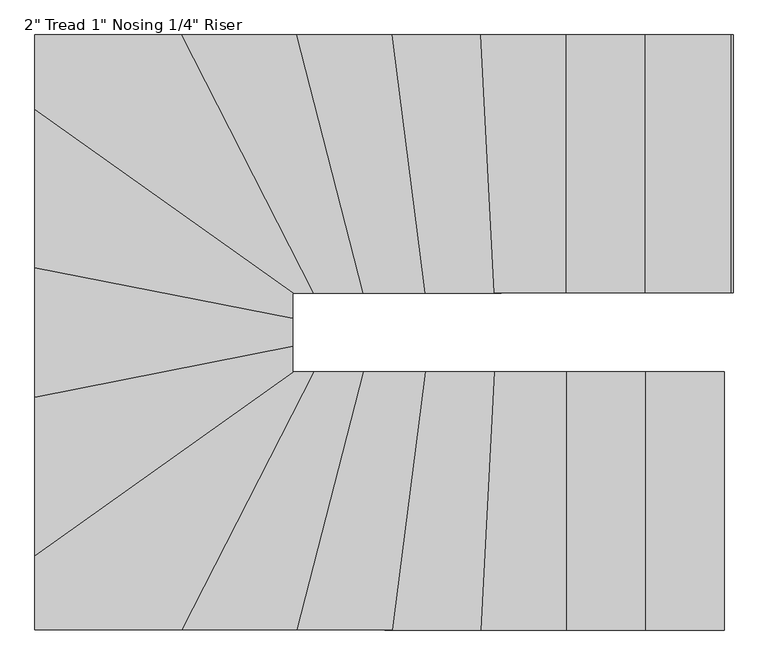
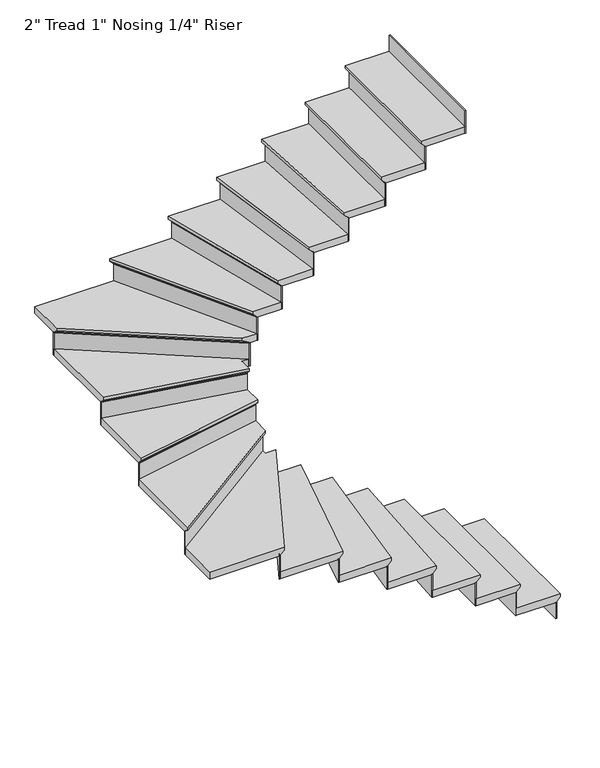
"""IFC4 building model written with IfcOpenShell, lengths in millimetres: stair flight geometry."""

from ifc_helpers import new_model, si_unit, origin, place, context, project, spatial, faceted_brep, source, transform, mapped, element, save


def stair_flight_e257120f(model_context):
    return source(origin(), model_context, "Body", "Brep", [
        faceted_brep([(-1783.4132248, -345.7070853, 3350.6833333), (-1783.4132248, -345.7070853, 3369.7333333), (-1783.4132248, -1260.1070853, 3369.7333333), (-1783.4132248, -1260.1070853, 3350.6833333), (-1808.8132248, -345.7070853, 3325.2833333), (-1808.8132248, -1260.1070853, 3325.2833333), (-2088.2132248, -345.7070853, 3369.7333333), (-2088.2132248, -1260.1070853, 3369.7333333), (-1808.8132248, -1260.1070853, 3318.9333333), (-2088.2132248, -1260.1070853, 3318.9333333), (-2088.2132248, -345.7070853, 3318.9333333), (-1808.8132248, -345.7070853, 3318.9333333)], [[[0, 1, 2, 3]], [[4, 0, 3, 5]], [[2, 1, 6, 7]], [[8, 9, 10, 11]], [[2, 7, 9, 8, 5, 3]], [[8, 11, 4, 5]], [[6, 1, 0, 4, 11, 10]], [[7, 6, 10, 9]]]),
        faceted_brep([(-1808.8132248, -345.7070853, 3318.9333333), (-1808.8132248, -345.7070853, 3200.4), (-1815.1632248, -345.7070853, 3200.4), (-1815.1632248, -345.7070853, 3318.9333333), (-1808.8132248, -1260.1070853, 3318.9333333), (-1815.1632248, -1260.1070853, 3318.9333333), (-1815.1632248, -1260.1070853, 3200.4), (-1808.8132248, -1260.1070853, 3200.4)], [[[0, 1, 2, 3]], [[4, 5, 6, 7]], [[1, 0, 4, 7]], [[2, 1, 7, 6]], [[3, 2, 6, 5]], [[0, 3, 5, 4]]]),
        faceted_brep([(-2088.2132248, -345.7070853, 3488.2666667), (-2088.2132248, -345.7070853, 3318.9333333), (-2094.5632248, -345.7070853, 3318.9333333), (-2094.5632248, -345.7070853, 3488.2666667), (-2088.2132248, -1260.1070853, 3488.2666667), (-2094.5632248, -1260.1070853, 3488.2666667), (-2094.5632248, -1260.1070853, 3318.9333333), (-2088.2132248, -1260.1070853, 3318.9333333)], [[[0, 1, 2, 3]], [[4, 5, 6, 7]], [[1, 0, 4, 7]], [[2, 1, 7, 6]], [[3, 2, 6, 5]], [[0, 3, 5, 4]]]),
        faceted_brep([(-2062.8132248, -1260.1070853, 3539.0666667), (-2062.8132248, -345.7070853, 3539.0666667), (-2367.6132248, -345.7070853, 3539.0666667), (-2367.6132248, -1260.1070853, 3539.0666667), (-2088.2132248, -1260.1070853, 3488.2666667), (-2367.6132248, -1260.1070853, 3488.2666667), (-2367.6132248, -345.7070853, 3488.2666667), (-2088.2132248, -345.7070853, 3488.2666667), (-2088.2132248, -1260.1070853, 3494.6166667), (-2062.8132248, -1260.1070853, 3520.0166667), (-2088.2132248, -345.7070853, 3494.6166667), (-2062.8132248, -345.7070853, 3520.0166667)], [[[0, 1, 2, 3]], [[4, 5, 6, 7]], [[0, 3, 5, 4, 8, 9]], [[4, 7, 10, 8]], [[2, 1, 11, 10, 7, 6]], [[3, 2, 6, 5]], [[11, 1, 0, 9]], [[10, 11, 9, 8]]]),
        faceted_brep([(-2367.6132248, -345.7070853, 3657.6), (-2367.6132248, -345.7070853, 3488.2666667), (-2373.9632248, -345.7070853, 3488.2666667), (-2373.9632248, -345.7070853, 3657.6), (-2367.6132248, -1260.1070853, 3657.6), (-2373.9632248, -1260.1070853, 3657.6), (-2373.9632248, -1260.1070853, 3488.2666667), (-2367.6132248, -1260.1070853, 3488.2666667)], [[[0, 1, 2, 3]], [[4, 5, 6, 7]], [[1, 0, 4, 7]], [[2, 1, 7, 6]], [[3, 2, 6, 5]], [[0, 3, 5, 4]]]),
        faceted_brep([(-2342.2132248, -1260.1070853, 3708.4), (-2342.2132248, -345.7070853, 3708.4), (-2623.2803863, -345.7070853, 3708.4), (-2670.8146567, -1260.1070853, 3708.4), (-2367.6132248, -1260.1070853, 3657.6), (-2670.8146567, -1260.1070853, 3657.6), (-2623.2803863, -345.7070853, 3657.6), (-2367.6132248, -345.7070853, 3657.6), (-2367.6132248, -1260.1070853, 3663.95), (-2342.2132248, -1260.1070853, 3689.35), (-2367.6132248, -345.7070853, 3663.95), (-2342.2132248, -345.7070853, 3689.35)], [[[0, 1, 2, 3]], [[4, 5, 6, 7]], [[0, 3, 5, 4, 8, 9]], [[4, 7, 10, 8]], [[2, 1, 11, 10, 7, 6]], [[3, 2, 6, 5]], [[11, 1, 0, 9]], [[10, 11, 9, 8]]]),
        faceted_brep([(-2623.2803863, -345.7070853, 3826.9333333), (-2623.2803863, -345.7070853, 3657.6), (-2629.6389604, -345.7070853, 3657.6), (-2629.6389604, -345.7070853, 3826.9333333), (-2670.8146567, -1260.1070853, 3826.9333333), (-2677.1732308, -1260.1070853, 3826.9333333), (-2677.1732308, -1260.1070853, 3657.6), (-2670.8146567, -1260.1070853, 3657.6)], [[[0, 1, 2, 3]], [[4, 5, 6, 7]], [[1, 0, 4, 7]], [[2, 1, 7, 6]], [[3, 2, 6, 5]], [[0, 3, 5, 4]]]),
        faceted_brep([(-2645.38036, -1260.1070853, 3877.7333333), (-2597.8460896, -345.7070853, 3877.7333333), (-2867.4470861, -345.7070853, 3877.7333333), (-2985.8031378, -1260.1070853, 3877.7333333), (-2670.8146567, -1260.1070853, 3826.9333333), (-2985.8031378, -1260.1070853, 3826.9333333), (-2867.4470861, -345.7070853, 3826.9333333), (-2623.2803863, -345.7070853, 3826.9333333), (-2670.8146567, -1260.1070853, 3833.2833333), (-2645.38036, -1260.1070853, 3858.6833333), (-2623.2803863, -345.7070853, 3833.2833333), (-2597.8460896, -345.7070853, 3858.6833333)], [[[0, 1, 2, 3]], [[4, 5, 6, 7]], [[0, 3, 5, 4, 8, 9]], [[4, 7, 10, 8]], [[2, 1, 11, 10, 7, 6]], [[3, 2, 6, 5]], [[11, 1, 0, 9]], [[10, 11, 9, 8]]]),
        faceted_brep([(-2867.4470861, -345.7070853, 3996.2666667), (-2867.4470861, -345.7070853, 3826.9333333), (-2873.8500579, -345.7070853, 3826.9333333), (-2873.8500579, -345.7070853, 3996.2666667), (-2985.8031378, -1260.1070853, 3996.2666667), (-2992.2061095, -1260.1070853, 3996.2666667), (-2992.2061095, -1260.1070853, 3826.9333333), (-2985.8031378, -1260.1070853, 3826.9333333)], [[[0, 1, 2, 3]], [[4, 5, 6, 7]], [[1, 0, 4, 7]], [[2, 1, 7, 6]], [[3, 2, 6, 5]], [[0, 3, 5, 4]]]),
        faceted_brep([(-2960.1912506, -1260.1070853, 4047.0666667), (-2841.835199, -345.7070853, 4047.0666667), (-3089.0743086, -345.7070853, 4047.0666667), (-3324.204756, -1260.1070853, 4047.0666667), (-2985.8031378, -1260.1070853, 3996.2666667), (-3324.204756, -1260.1070853, 3996.2666667), (-3089.0743086, -345.7070853, 3996.2666667), (-2867.4470861, -345.7070853, 3996.2666667), (-2985.8031378, -1260.1070853, 4002.6166667), (-2960.1912506, -1260.1070853, 4028.0166667), (-2867.4470861, -345.7070853, 4002.6166667), (-2841.835199, -345.7070853, 4028.0166667)], [[[0, 1, 2, 3]], [[4, 5, 6, 7]], [[0, 3, 5, 4, 8, 9]], [[4, 7, 10, 8]], [[2, 1, 11, 10, 7, 6]], [[3, 2, 6, 5]], [[11, 1, 0, 9]], [[10, 11, 9, 8]]]),
        faceted_brep([(-3089.0743086, -345.7070853, 4165.6), (-3089.0743086, -345.7070853, 3996.2666667), (-3095.6308854, -345.7070853, 3996.2666667), (-3095.6308854, -345.7070853, 4165.6), (-3324.204756, -1260.1070853, 4165.6), (-3330.7613329, -1260.1070853, 4165.6), (-3330.7613329, -1260.1070853, 3996.2666667), (-3324.204756, -1260.1070853, 3996.2666667)], [[[0, 1, 2, 3]], [[4, 5, 6, 7]], [[1, 0, 4, 7]], [[2, 1, 7, 6]], [[3, 2, 6, 5]], [[0, 3, 5, 4]]]),
        faceted_brep([(-3297.9784485, -1260.1070853, 4216.4), (-3062.8480011, -345.7070853, 4216.4), (-3265.4209447, -345.7070853, 4216.4), (-3734.245566, -1260.1070853, 4216.4), (-3324.204756, -1260.1070853, 4165.6), (-3734.245566, -1260.1070853, 4165.6), (-3265.4209447, -345.7070853, 4165.6), (-3089.0743086, -345.7070853, 4165.6), (-3324.204756, -1260.1070853, 4171.95), (-3297.9784485, -1260.1070853, 4197.35), (-3089.0743086, -345.7070853, 4171.95), (-3062.8480011, -345.7070853, 4197.35)], [[[0, 1, 2, 3]], [[4, 5, 6, 7]], [[0, 3, 5, 4, 8, 9]], [[4, 7, 10, 8]], [[2, 1, 11, 10, 7, 6]], [[3, 2, 6, 5]], [[11, 1, 0, 9]], [[10, 11, 9, 8]]]),
        faceted_brep([(-3265.4209447, -345.7070853, 4334.9333333), (-3265.4209447, -345.7070853, 4165.6), (-3272.5569278, -345.7070853, 4165.6), (-3272.5569278, -345.7070853, 4334.9333333), (-3734.245566, -1260.1070853, 4334.9333333), (-3741.3815491, -1260.1070853, 4334.9333333), (-3741.3815491, -1260.1070853, 4165.6), (-3734.245566, -1260.1070853, 4165.6)], [[[0, 1, 2, 3]], [[4, 5, 6, 7]], [[1, 0, 4, 7]], [[2, 1, 7, 6]], [[3, 2, 6, 5]], [[0, 3, 5, 4]]]),
        faceted_brep([(-4225.5449167, -966.4259516, 4385.7333333), (-4225.5449167, -1260.1070853, 4385.7333333), (-3705.7016335, -1260.1070853, 4385.7333333), (-3236.8770121, -345.7070853, 4385.7333333), (-3311.1449167, -345.7070853, 4385.7333333), (-3311.1449167, -316.1520025, 4385.7333333), (-4225.5449167, -1260.1070853, 4334.9333333), (-4225.5449167, -966.4259516, 4334.9333333), (-3311.1449167, -316.1520025, 4334.9333333), (-3311.1449167, -345.7070853, 4334.9333333), (-3265.4209447, -345.7070853, 4334.9333333), (-3734.245566, -1260.1070853, 4334.9333333), (-3734.245566, -1260.1070853, 4341.2833333), (-3705.7016335, -1260.1070853, 4366.6833333), (-3265.4209447, -345.7070853, 4341.2833333), (-3236.8770121, -345.7070853, 4366.6833333)], [[[0, 1, 2, 3, 4, 5]], [[6, 7, 8, 9, 10, 11]], [[1, 0, 7, 6]], [[2, 1, 6, 11, 12, 13]], [[11, 10, 14, 12]], [[4, 3, 15, 14, 10, 9]], [[5, 4, 9, 8]], [[0, 5, 8, 7]], [[15, 3, 2, 13]], [[14, 15, 13, 12]]]),
        faceted_brep([(-3311.1449167, -316.1520025, 4504.2666667), (-3311.1449167, -316.1520025, 4334.9333333), (-3311.1449167, -308.3600277, 4334.9333333), (-3311.1449167, -308.3600277, 4504.2666667), (-4225.5449167, -966.4259516, 4504.2666667), (-4225.5449167, -958.6339768, 4504.2666667), (-4225.5449167, -958.6339768, 4334.9333333), (-4225.5449167, -966.4259516, 4334.9333333)], [[[0, 1, 2, 3]], [[4, 5, 6, 7]], [[1, 0, 4, 7]], [[2, 1, 7, 6]], [[3, 2, 6, 5]], [[0, 3, 5, 4]]]),
        faceted_brep([(-4225.5449167, -997.5938508, 4555.0666667), (-3311.1449167, -347.3199017, 4555.0666667), (-3311.1449167, -229.6979154, 4555.0666667), (-4225.5449167, -409.9387717, 4555.0666667), (-4225.5449167, -966.4259516, 4504.2666667), (-4225.5449167, -409.9387717, 4504.2666667), (-3311.1449167, -229.6979154, 4504.2666667), (-3311.1449167, -316.1520025, 4504.2666667), (-4225.5449167, -966.4259516, 4510.6166667), (-4225.5449167, -997.5938508, 4536.0166667), (-3311.1449167, -316.1520025, 4510.6166667), (-3311.1449167, -347.3199017, 4536.0166667)], [[[0, 1, 2, 3]], [[4, 5, 6, 7]], [[0, 3, 5, 4, 8, 9]], [[4, 7, 10, 8]], [[2, 1, 11, 10, 7, 6]], [[3, 2, 6, 5]], [[11, 1, 0, 9]], [[10, 11, 9, 8]]]),
        faceted_brep([(-3311.1449167, -229.6979154, 4673.6), (-3311.1449167, -229.6979154, 4504.2666667), (-3311.1449167, -223.22573, 4504.2666667), (-3311.1449167, -223.22573, 4673.6), (-4225.5449167, -409.9387717, 4673.6), (-4225.5449167, -403.4665863, 4673.6), (-4225.5449167, -403.4665863, 4504.2666667), (-4225.5449167, -409.9387717, 4504.2666667)], [[[0, 1, 2, 3]], [[4, 5, 6, 7]], [[1, 0, 4, 7]], [[2, 1, 7, 6]], [[3, 2, 6, 5]], [[0, 3, 5, 4]]]),
        faceted_brep([(-4225.5449167, -435.8275135, 4724.4), (-3311.1449167, -255.5866572, 4724.4), (-3311.1449167, -130.5387717, 4724.4), (-4225.5449167, 49.7020846, 4724.4), (-4225.5449167, -409.9387717, 4673.6), (-4225.5449167, 49.7020846, 4673.6), (-3311.1449167, -130.5387717, 4673.6), (-3311.1449167, -229.6979154, 4673.6), (-4225.5449167, -409.9387717, 4679.95), (-4225.5449167, -435.8275135, 4705.35), (-3311.1449167, -229.6979154, 4679.95), (-3311.1449167, -255.5866572, 4705.35)], [[[0, 1, 2, 3]], [[4, 5, 6, 7]], [[0, 3, 5, 4, 8, 9]], [[4, 7, 10, 8]], [[2, 1, 11, 10, 7, 6]], [[3, 2, 6, 5]], [[11, 1, 0, 9]], [[10, 11, 9, 8]]]),
        faceted_brep([(-3311.1449167, -130.5387717, 4842.9333333), (-3311.1449167, -130.5387717, 4673.6), (-3311.1449167, -124.0665863, 4673.6), (-3311.1449167, -124.0665863, 4842.9333333), (-4225.5449167, 49.7020846, 4842.9333333), (-4225.5449167, 56.17427, 4842.9333333), (-4225.5449167, 56.17427, 4673.6), (-4225.5449167, 49.7020846, 4673.6)], [[[0, 1, 2, 3]], [[4, 5, 6, 7]], [[1, 0, 4, 7]], [[2, 1, 7, 6]], [[3, 2, 6, 5]], [[0, 3, 5, 4]]]),
        faceted_brep([(-4225.5449167, 23.8133428, 4893.7333333), (-3311.1449167, -156.4275135, 4893.7333333), (-3311.1449167, -66.3070853, 4893.7333333), (-3265.0494422, -66.3070853, 4893.7333333), (-4225.5449167, 616.7475793, 4893.7333333), (-4225.5449167, 49.7020846, 4842.9333333), (-4225.5449167, 616.7475793, 4842.9333333), (-3265.0494422, -66.3070853, 4842.9333333), (-3311.1449167, -66.3070853, 4842.9333333), (-3311.1449167, -130.5387717, 4842.9333333), (-4225.5449167, 49.7020846, 4849.2833333), (-4225.5449167, 23.8133428, 4874.6833333), (-3311.1449167, -130.5387717, 4849.2833333), (-3311.1449167, -156.4275135, 4874.6833333)], [[[0, 1, 2, 3, 4]], [[5, 6, 7, 8, 9]], [[0, 4, 6, 5, 10, 11]], [[5, 9, 12, 10]], [[2, 1, 13, 12, 9, 8]], [[3, 2, 8, 7]], [[4, 3, 7, 6]], [[13, 1, 0, 11]], [[12, 13, 11, 10]]]),
        faceted_brep([(-3265.0494422, -66.3070853, 5012.2666667), (-3265.0494422, -66.3070853, 4842.9333333), (-3254.0925497, -66.3070853, 4842.9333333), (-3254.0925497, -66.3070853, 5012.2666667), (-4225.5449167, 616.7475793, 5012.2666667), (-4225.5449167, 624.5395541, 5012.2666667), (-4225.5449167, 624.5395541, 4842.9333333), (-4225.5449167, 616.7475793, 4842.9333333)], [[[0, 1, 2, 3]], [[4, 5, 6, 7]], [[1, 0, 4, 7]], [[2, 1, 7, 6]], [[3, 2, 6, 5]], [[0, 3, 5, 4]]]),
        faceted_brep([(-3677.1577009, 848.0929147, 5063.0666667), (-4225.5449167, 848.0929147, 5063.0666667), (-4225.5449167, 585.5796802, 5063.0666667), (-3308.8770121, -66.3070853, 5063.0666667), (-3208.3330796, -66.3070853, 5063.0666667), (-4225.5449167, 848.0929147, 5012.2666667), (-3677.1577009, 848.0929147, 5012.2666667), (-3208.3330796, -66.3070853, 5012.2666667), (-3265.0494422, -66.3070853, 5012.2666667), (-4225.5449167, 616.7475793, 5012.2666667), (-4225.5449167, 616.7475793, 5018.6166667), (-4225.5449167, 585.5796802, 5044.0166667), (-3265.0494422, -66.3070853, 5018.6166667), (-3308.8770121, -66.3070853, 5044.0166667)], [[[0, 1, 2, 3, 4]], [[5, 6, 7, 8, 9]], [[1, 0, 6, 5]], [[2, 1, 5, 9, 10, 11]], [[9, 8, 12, 10]], [[4, 3, 13, 12, 8, 7]], [[0, 4, 7, 6]], [[13, 3, 2, 11]], [[12, 13, 11, 10]]]),
        faceted_brep([(-3208.3330796, -66.3070853, 5181.6), (-3208.3330796, -66.3070853, 5012.2666667), (-3201.1970965, -66.3070853, 5012.2666667), (-3201.1970965, -66.3070853, 5181.6), (-3677.1577009, 848.0929147, 5181.6), (-3670.0217178, 848.0929147, 5181.6), (-3670.0217178, 848.0929147, 5012.2666667), (-3677.1577009, 848.0929147, 5012.2666667)], [[[0, 1, 2, 3]], [[4, 5, 6, 7]], [[1, 0, 4, 7]], [[2, 1, 7, 6]], [[3, 2, 6, 5]], [[0, 3, 5, 4]]]),
        faceted_brep([(-3705.7016335, 848.0929147, 5232.4), (-3236.8770121, -66.3070853, 5232.4), (-3036.6216937, -66.3070853, 5232.4), (-3271.7521411, 848.0929147, 5232.4), (-3677.1577009, 848.0929147, 5181.6), (-3271.7521411, 848.0929147, 5181.6), (-3036.6216937, -66.3070853, 5181.6), (-3208.3330796, -66.3070853, 5181.6), (-3677.1577009, 848.0929147, 5187.95), (-3705.7016335, 848.0929147, 5213.35), (-3208.3330796, -66.3070853, 5187.95), (-3236.8770121, -66.3070853, 5213.35)], [[[0, 1, 2, 3]], [[4, 5, 6, 7]], [[0, 3, 5, 4, 8, 9]], [[4, 7, 10, 8]], [[2, 1, 11, 10, 7, 6]], [[3, 2, 6, 5]], [[11, 1, 0, 9]], [[10, 11, 9, 8]]]),
        faceted_brep([(-3036.6216937, -66.3070853, 5350.9333333), (-3036.6216937, -66.3070853, 5181.6), (-3030.0651168, -66.3070853, 5181.6), (-3030.0651168, -66.3070853, 5350.9333333), (-3271.7521411, 848.0929147, 5350.9333333), (-3265.1955642, 848.0929147, 5350.9333333), (-3265.1955642, 848.0929147, 5181.6), (-3271.7521411, 848.0929147, 5181.6)], [[[0, 1, 2, 3]], [[4, 5, 6, 7]], [[1, 0, 4, 7]], [[2, 1, 7, 6]], [[3, 2, 6, 5]], [[0, 3, 5, 4]]]),
        faceted_brep([(-3297.9784485, 848.0929147, 5401.7333333), (-3062.8480011, -66.3070853, 5401.7333333), (-2816.2233119, -66.3070853, 5401.7333333), (-2934.5793635, 848.0929147, 5401.7333333), (-3271.7521411, 848.0929147, 5350.9333333), (-2934.5793635, 848.0929147, 5350.9333333), (-2816.2233119, -66.3070853, 5350.9333333), (-3036.6216937, -66.3070853, 5350.9333333), (-3271.7521411, 848.0929147, 5357.2833333), (-3297.9784485, 848.0929147, 5382.6833333), (-3036.6216937, -66.3070853, 5357.2833333), (-3062.8480011, -66.3070853, 5382.6833333)], [[[0, 1, 2, 3]], [[4, 5, 6, 7]], [[0, 3, 5, 4, 8, 9]], [[4, 7, 10, 8]], [[2, 1, 11, 10, 7, 6]], [[3, 2, 6, 5]], [[11, 1, 0, 9]], [[10, 11, 9, 8]]]),
        faceted_brep([(-2816.2233119, -66.3070853, 5520.2666667), (-2816.2233119, -66.3070853, 5350.9333333), (-2809.8203401, -66.3070853, 5350.9333333), (-2809.8203401, -66.3070853, 5520.2666667), (-2934.5793635, 848.0929147, 5520.2666667), (-2928.1763918, 848.0929147, 5520.2666667), (-2928.1763918, 848.0929147, 5350.9333333), (-2934.5793635, 848.0929147, 5350.9333333)], [[[0, 1, 2, 3]], [[4, 5, 6, 7]], [[1, 0, 4, 7]], [[2, 1, 7, 6]], [[3, 2, 6, 5]], [[0, 3, 5, 4]]]),
        faceted_brep([(-2960.1912506, 848.0929147, 5571.0666667), (-2841.835199, -66.3070853, 5571.0666667), (-2572.411793, -66.3070853, 5571.0666667), (-2619.9460634, 848.0929147, 5571.0666667), (-2934.5793635, 848.0929147, 5520.2666667), (-2619.9460634, 848.0929147, 5520.2666667), (-2572.411793, -66.3070853, 5520.2666667), (-2816.2233119, -66.3070853, 5520.2666667), (-2934.5793635, 848.0929147, 5526.6166667), (-2960.1912506, 848.0929147, 5552.0166667), (-2816.2233119, -66.3070853, 5526.6166667), (-2841.835199, -66.3070853, 5552.0166667)], [[[0, 1, 2, 3]], [[4, 5, 6, 7]], [[0, 3, 5, 4, 8, 9]], [[4, 7, 10, 8]], [[2, 1, 11, 10, 7, 6]], [[3, 2, 6, 5]], [[11, 1, 0, 9]], [[10, 11, 9, 8]]]),
        faceted_brep([(-2572.411793, -66.3070853, 5689.6), (-2572.411793, -66.3070853, 5520.2666667), (-2566.0532188, -66.3070853, 5520.2666667), (-2566.0532188, -66.3070853, 5689.6), (-2619.9460634, 848.0929147, 5689.6), (-2613.5874892, 848.0929147, 5689.6), (-2613.5874892, 848.0929147, 5520.2666667), (-2619.9460634, 848.0929147, 5520.2666667)], [[[0, 1, 2, 3]], [[4, 5, 6, 7]], [[1, 0, 4, 7]], [[2, 1, 7, 6]], [[3, 2, 6, 5]], [[0, 3, 5, 4]]]),
        faceted_brep([(-2645.38036, 848.0929147, 5740.4), (-2597.8460896, -66.3070853, 5740.4), (-2316.8132248, -66.3070853, 5740.4), (-2316.8132248, 848.0929147, 5740.4), (-2619.9460634, 848.0929147, 5689.6), (-2316.8132248, 848.0929147, 5689.6), (-2316.8132248, -66.3070853, 5689.6), (-2572.411793, -66.3070853, 5689.6), (-2619.9460634, 848.0929147, 5695.95), (-2645.38036, 848.0929147, 5721.35), (-2572.411793, -66.3070853, 5695.95), (-2597.8460896, -66.3070853, 5721.35)], [[[0, 1, 2, 3]], [[4, 5, 6, 7]], [[0, 3, 5, 4, 8, 9]], [[4, 7, 10, 8]], [[2, 1, 11, 10, 7, 6]], [[3, 2, 6, 5]], [[11, 1, 0, 9]], [[10, 11, 9, 8]]]),
        faceted_brep([(-2316.8132248, -66.3070853, 5858.9333333), (-2316.8132248, -66.3070853, 5689.6), (-2310.4632248, -66.3070853, 5689.6), (-2310.4632248, -66.3070853, 5858.9333333), (-2316.8132248, 848.0929147, 5858.9333333), (-2310.4632248, 848.0929147, 5858.9333333), (-2310.4632248, 848.0929147, 5689.6), (-2316.8132248, 848.0929147, 5689.6)], [[[0, 1, 2, 3]], [[4, 5, 6, 7]], [[1, 0, 4, 7]], [[2, 1, 7, 6]], [[3, 2, 6, 5]], [[0, 3, 5, 4]]]),
        faceted_brep([(-2342.2132248, 848.0929147, 5909.7333333), (-2342.2132248, -66.3070853, 5909.7333333), (-2037.4132248, -66.3070853, 5909.7333333), (-2037.4132248, 848.0929147, 5909.7333333), (-2316.8132248, 848.0929147, 5858.9333333), (-2037.4132248, 848.0929147, 5858.9333333), (-2037.4132248, -66.3070853, 5858.9333333), (-2316.8132248, -66.3070853, 5858.9333333), (-2316.8132248, 848.0929147, 5865.2833333), (-2342.2132248, 848.0929147, 5890.6833333), (-2316.8132248, -66.3070853, 5865.2833333), (-2342.2132248, -66.3070853, 5890.6833333)], [[[0, 1, 2, 3]], [[4, 5, 6, 7]], [[0, 3, 5, 4, 8, 9]], [[4, 7, 10, 8]], [[2, 1, 11, 10, 7, 6]], [[3, 2, 6, 5]], [[11, 1, 0, 9]], [[10, 11, 9, 8]]]),
        faceted_brep([(-2037.4132248, -66.3070853, 6028.2666667), (-2037.4132248, -66.3070853, 5858.9333333), (-2031.0632248, -66.3070853, 5858.9333333), (-2031.0632248, -66.3070853, 6028.2666667), (-2037.4132248, 848.0929147, 6028.2666667), (-2031.0632248, 848.0929147, 6028.2666667), (-2031.0632248, 848.0929147, 5858.9333333), (-2037.4132248, 848.0929147, 5858.9333333)], [[[0, 1, 2, 3]], [[4, 5, 6, 7]], [[1, 0, 4, 7]], [[2, 1, 7, 6]], [[3, 2, 6, 5]], [[0, 3, 5, 4]]]),
        faceted_brep([(-1758.0132248, -66.3070853, 6197.6), (-1758.0132248, -66.3070853, 6028.2666667), (-1751.6632248, -66.3070853, 6028.2666667), (-1751.6632248, -66.3070853, 6197.6), (-1758.0132248, 848.0929147, 6197.6), (-1751.6632248, 848.0929147, 6197.6), (-1751.6632248, 848.0929147, 6028.2666667), (-1758.0132248, 848.0929147, 6028.2666667)], [[[0, 1, 2, 3]], [[4, 5, 6, 7]], [[1, 0, 4, 7]], [[2, 1, 7, 6]], [[3, 2, 6, 5]], [[0, 3, 5, 4]]]),
        faceted_brep([(-2062.8132248, 848.0929147, 6079.0666667), (-2062.8132248, -66.3070853, 6079.0666667), (-1758.0132248, -66.3070853, 6079.0666667), (-1758.0132248, 848.0929147, 6079.0666667), (-2037.4132248, 848.0929147, 6028.2666667), (-1758.0132248, 848.0929147, 6028.2666667), (-1758.0132248, -66.3070853, 6028.2666667), (-2037.4132248, -66.3070853, 6028.2666667), (-2037.4132248, 848.0929147, 6034.6166667), (-2062.8132248, 848.0929147, 6060.0166667), (-2037.4132248, -66.3070853, 6034.6166667), (-2062.8132248, -66.3070853, 6060.0166667)], [[[0, 1, 2, 3]], [[4, 5, 6, 7]], [[0, 3, 5, 4, 8, 9]], [[4, 7, 10, 8]], [[2, 1, 11, 10, 7, 6]], [[3, 2, 6, 5]], [[11, 1, 0, 9]], [[10, 11, 9, 8]]]),
    ])


if __name__ == "__main__":
    model = new_model("IFC4")
    model_context = context("Model", 3, world=origin())
    ifc_project = project(units=[si_unit("LENGTHUNIT", "METRE", prefix="MILLI")], contexts=[model_context])
    site = spatial("IfcSite", under=ifc_project)
    building = spatial("IfcBuilding", under=site)
    placement = place(None, origin())
    stair_flight_shape = stair_flight_e257120f(model_context)
    element("IfcStairFlight", 1, ObjectType="2\" Tread 1\" Nosing 1/4\" Riser", at=placement, inside=building, context=model_context, shape_type="MappedRepresentation", body=[
        mapped(stair_flight_shape, transform((0.0, 0.0, 0.0), x_axis=(1.0, 0.0, 0.0), y_axis=(0.0, 1.0, 0.0), z_axis=(0.0, 0.0, 1.0))),
    ])
    save(model, "model.ifc")
